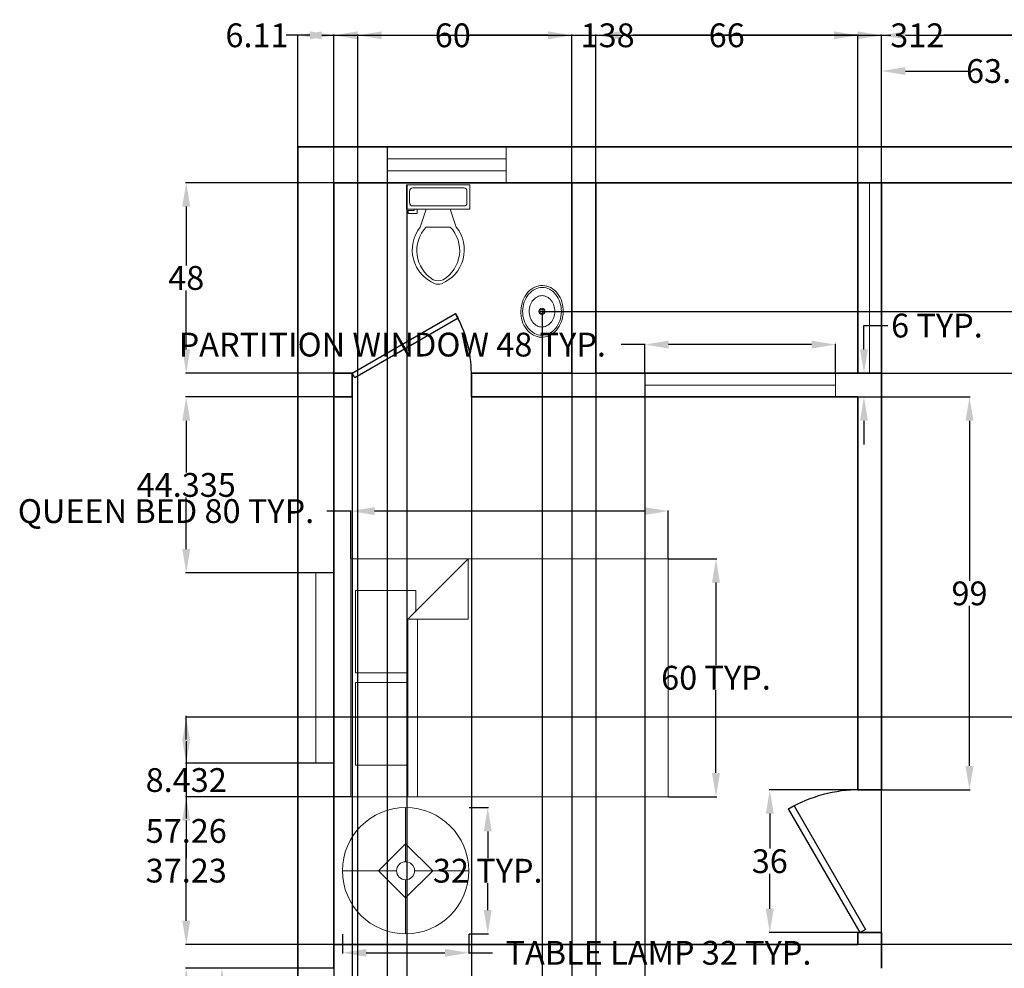
# Model space of a CAD drawing. Units: inches. Extents: x 351 to 774, y 111 to 703.
# Tile 5 of 6: x 351 to 599, y 464 to 703. Entities that reach past the tile are written whole.
import ezdxf

# ---------------------------------------------------------------- set-up
doc = ezdxf.new("R2010")
doc.units = ezdxf.units.IN
doc.header["$MEASUREMENT"] = 0
for name, color, linetype, lineweight in [('A-ANNO-DIMS', 2, 'Continuous', 18), ('A-DOOR', 3, 'Continuous', 25), ('A-FLOR-FIXT', 9, 'Continuous', 18), ('A-FURN', 8, 'Continuous', 18), ('A-GLAZ', 4, 'Continuous', 18), ('A-WALL', 7, 'Continuous', 35)]:
    doc.layers.add(name, color=color, linetype=linetype, lineweight=lineweight)
doc.styles.get("Standard").update_dxf_attribs({"font": 'arial.ttf'})
doc.dimstyles.get("Standard").update_dxf_attribs({"dimtxt": 6, "dimasz": 6, "dimexe": 0.18, "dimexo": 0.0625, "dimgap": 0.09, "dimtad": 0, "dimtih": 1, "dimtoh": 1, "dimdec": 0, "dimzin": 0, "dimdsep": 46, "dimlunit": 3, "dimtxsty": 'Standard', "dimcen": 0.09, "dimadec": 0, "dimazin": 0, "dimtfac": 1, "dimtdec": 0, "dimtofl": 0, "dimtmove": 0, "dimatfit": 3, "dimfxl": 1, "dimtolj": 1, "dimtzin": 0, "dimarcsym": 0})

# ---------------------------------------------------------------- blocks, each defined once
blk = doc.blocks.new('*U3')
for p, q in [((0, 0), (0, -6)), ((40, 0), (40, -6))]:
    blk.add_line(p, q)
blk.add_lwpolyline([(0, 0), (34.64, 20), (35.52, 18.48), (0.88, -1.52)], close=True)
blk.add_arc((0, 0), 40, 0, 30)
blk = doc.blocks.new('*U4')
for p, q in [((-40, 0), (-40, 6)), ((0, 0), (0, 6))]:
    blk.add_line(p, q)
blk.add_lwpolyline([(0, 0), (-34.64, -20), (-35.52, -18.48), (-0.88, 1.52)], close=True)
blk.add_arc((0, 0), 40, 180, 210)
blk = doc.blocks.new('Bed - Queen')
for p, q in [((0, -80.00003), (0, 0)), ((0, 0), (59.99999, 0)), ((59.99999, 0), (59.99999, -80.00003)), ((7.99999, -1.2), (28.79998, -1.2)), ((7.99999, -14.4), (7.99999, -1.2)), ((28.79998, -1.2), (28.79998, -14.4)), ((31.19999, -1.2), (51.99999, -1.2)), ((31.19999, -14.4), (31.19999, -1.2)), ((51.99999, -1.2), (51.99999, -16.4)), ((0, -14.4), (44.8, -14.4)), ((59.99999, -29.6), (44.8, -14.4)), ((44.8, -14.4), (44.8, -29.6)), ((44.8, -16.8), (0, -16.8)), ((51.99999, -16.4), (46.79936, -16.4)), ((44.8, -29.6), (59.99999, -29.6)), ((59.99999, -80.00003), (0, -80.00003))]:
    blk.add_line(p, q)
blk = doc.blocks.new('Lamp - Table')
for p, q in [((0, 7), (0, 1)), ((0, 3), (-3, 0)), ((3, 0), (0, 3)), ((-1, 0), (-7, 0)), ((-3, 0), (0, -3)), ((0, -3), (3, 0)), ((1, 0), (7, 0)), ((0, -1), (0, -7))]:
    blk.add_line(p, q)
for radius in [7, 1]:
    blk.add_circle((0, 0), radius)
blk = doc.blocks.new('Toilet - top')
for p, q in [((9.5, -6), (9.5, -2)), ((-10, -8.5), (-8, -8.5)), ((-10, -9.5), (-10, -8.5)), ((-7, -9.5), (-10, -9.5)), ((-8, -8.5), (-8, -8)), ((-7, -8), (-7, -9.5)), ((-4, -8), (-6, -14)), ((4, -8), (6, -14)), ((4, -14), (-4, -14))]:
    blk.add_line(p, q)
blk.add_lwpolyline([(10.5, -8), (10.5, 0), (-10.5, 0), (-10.5, -8)], close=True)
for points in [[(-9.5, -2), (-9.5, -6)], [(8.5, -1), (-8.5, -1)], [(-8.5, -7), (8.5, -7)]]:
    blk.add_lwpolyline(points)
for centre, radius, start, end in [((-8.62, -1.88), 0.884, 81.8699, 188.1301), ((8.62, -1.88), 0.884, 351.8699, 98.1301), ((-8.62, -6.12), 0.884, 171.8699, 278.1301), ((8.62, -6.12), 0.884, 261.8699, 8.1301), ((3.52, -21.58), 12.17, 141.4691, 247.9714), ((4.2, -21.82), 11.33, 136.3677, 238.9468), ((-3.52, -21.58), 12.17, 292.0284, 38.5307), ((-4.2, -21.82), 11.33, 301.053, 43.6321), ((0, -27.88), 4, 245.7318, 294.2682), ((0, -29), 4, 254.8605, 285.1395)]:
    blk.add_arc(centre, radius, start, end)
blk = doc.blocks.new('Sink - Oval top')
for p, q in [((-1, 0), (1, 0)), ((0, 1), (0, -1))]:
    blk.add_line(p, q)
for points in [[(-12.23, 0.39, 0.117634), (-11.46, -3.36, 0.104469), (-8.88, -6.8, 0.090016), (-5.08, -9.07, 0.08192), (-0.32, -10.02, 0.08192), (4.49, -9.38, 0.090016), (8.42, -7.36, 0.104469), (11.22, -4.09, 0.117634), (12.23, -0.39, 0.117634), (11.46, 3.36, 0.104469), (8.88, 6.8, 0.090016), (5.08, 9.07, 0.08192), (0.32, 10.02, 0.08192), (-4.49, 9.38, 0.090016), (-8.42, 7.36, 0.104469), (-11.22, 4.09, 0.117634)], [(-11.29, 0.16, 0.118622), (-10.52, -3.25, 0.104678), (-8.07, -6.36, 0.089562), (-4.54, -8.37, 0.081185), (-0.13, -9.15, 0.081185), (4.3, -8.49, 0.089562), (7.89, -6.58, 0.104678), (10.42, -3.55, 0.118622), (11.29, -0.16, 0.118622), (10.52, 3.25, 0.104678), (8.07, 6.36, 0.089562), (4.54, 8.37, 0.081185), (0.13, 9.15, 0.081185), (-4.3, 8.49, 0.089562), (-7.89, 6.58, 0.104678), (-10.42, 3.55, 0.118622)], [(-7.42, 0.08, 0.118283), (-6.91, -2.17, 0.104607), (-5.29, -4.21, 0.089718), (-2.97, -5.53, 0.081436), (-0.07, -6.04, 0.081436), (2.84, -5.59, 0.089718), (5.2, -4.33, 0.104607), (6.86, -2.32, 0.118283), (7.42, -0.08, 0.118283), (6.91, 2.17, 0.104607), (5.29, 4.21, 0.089718), (2.97, 5.53, 0.081436), (0.07, 6.04, 0.081436), (-2.84, 5.59, 0.089718), (-5.2, 4.33, 0.104607), (-6.86, 2.32, 0.118283)]]:
    blk.add_lwpolyline(points, format="xyb", close=True)
for radius in [1.5, 1]:
    blk.add_circle((0, 0), radius)
blk = doc.blocks.new('WIN-48IN-6IN-WALL')
blk.add_line((3, 48), (3, 0))
blk.add_lwpolyline([(0, 48), (6, 48), (6, 0), (0, 0)], close=True)
blk = doc.blocks.new('WIN-48IN-9IN-WALL')
blk.add_line((4.5, 48), (4.5, 0))
blk.add_lwpolyline([(0, 0), (9, 0), (9, 48), (0, 48)], close=True)
blk = doc.blocks.new('WIN-BATH-30IN-9IN-WALL')
for p, q in [((0, 0), (0, 9)), ((0, 9), (30, 9)), ((30, 9), (30, 0)), ((0, 6), (30, 6)), ((30, 3), (0, 3)), ((30, 0), (0, 0))]:
    blk.add_line(p, q)
blk = doc.blocks.new('*D22')
at = {"layer": 'A-ANNO-DIMS', "color": 0, "lineweight": -2, "transparency": 16777216}
for p, q in [((508.41, 621.44), (502.41, 621.44)), ((508.41, 614.3), (508.41, 621.62)), ((550.41, 621.44), (514.41, 621.44)), ((556.41, 614.3), (556.41, 621.62))]:
    blk.add_line(p, q, dxfattribs=at)
at = {"layer": 'A-ANNO-DIMS', "color": 0, "transparency": 16777216}
for points in [[(514.41, 622.44), (514.41, 620.44), (508.41, 621.44)], [(550.41, 622.44), (550.41, 620.44), (556.41, 621.44)]]:
    blk.add_solid(points, dxfattribs=at)
at = {"layer": 'Defpoints', "color": 0, "transparency": 16777216}
for p in [(508.41, 621.44), (508.41, 614.24), (556.41, 614.24)]:
    blk.add_point(p, dxfattribs=at)
at = {"layer": 'A-ANNO-DIMS', "color": 0, "transparency": 16777216, "insert": (444.8, 621.44), "char_height": 6, "attachment_point": 5}
blk.add_mtext('\\A1;PARTITION WINDOW 48 TYP.', dxfattribs=at)
blk = doc.blocks.new('*D23')
at = {"layer": 'A-ANNO-DIMS', "color": 0, "lineweight": -2, "transparency": 16777216}
for p, q in [((563.61, 620.24), (563.61, 626.24)), ((563.61, 626.24), (569.61, 626.24)), ((556.48, 614.24), (563.79, 614.24)), ((556.48, 608.24), (563.79, 608.24)), ((563.61, 602.24), (563.61, 596.24))]:
    blk.add_line(p, q, dxfattribs=at)
at = {"layer": 'A-ANNO-DIMS', "color": 0, "transparency": 16777216}
for points in [[(562.61, 620.24), (564.61, 620.24), (563.61, 614.24)], [(562.61, 602.24), (564.61, 602.24), (563.61, 608.24)]]:
    blk.add_solid(points, dxfattribs=at)
at = {"layer": 'Defpoints', "color": 0, "transparency": 16777216}
for p in [(556.41, 614.24), (563.61, 614.24), (556.41, 608.24)]:
    blk.add_point(p, dxfattribs=at)
at = {"layer": 'A-ANNO-DIMS', "color": 0, "transparency": 16777216, "insert": (581.99, 626.24), "char_height": 6, "attachment_point": 5}
blk.add_mtext('\\A1;6 TYP.', dxfattribs=at)
blk = doc.blocks.new('*D28')
at = {"layer": 'A-ANNO-DIMS', "color": 0, "lineweight": -2, "transparency": 16777216}
for p, q in [((432.23, 472.86), (432.23, 467.97)), ((464.06, 472.86), (464.06, 467.97)), ((438.23, 468.15), (458.06, 468.15)), ((464.06, 468.15), (470.06, 468.15))]:
    blk.add_line(p, q, dxfattribs=at)
at = {"layer": 'A-ANNO-DIMS', "color": 0, "transparency": 16777216}
for points in [[(438.23, 469.15), (438.23, 467.15), (432.23, 468.15)], [(458.06, 469.15), (458.06, 467.15), (464.06, 468.15)]]:
    blk.add_solid(points, dxfattribs=at)
at = {"layer": 'Defpoints', "color": 0, "transparency": 16777216}
for p in [(432.23, 472.92), (464.06, 472.92), (464.06, 468.15)]:
    blk.add_point(p, dxfattribs=at)
at = {"layer": 'A-ANNO-DIMS', "color": 0, "transparency": 16777216, "insert": (511.85, 468.15), "char_height": 6, "attachment_point": 5}
blk.add_mtext('\\A1;TABLE LAMP 32 TYP.', dxfattribs=at)
blk = doc.blocks.new('*D29')
at = {"layer": 'A-ANNO-DIMS', "color": 0, "lineweight": -2, "transparency": 16777216}
for p, q in [((464.12, 504.75), (469.02, 504.75)), ((468.84, 498.75), (468.84, 491.99)), ((468.84, 478.92), (468.84, 485.68)), ((464.12, 472.92), (469.02, 472.92))]:
    blk.add_line(p, q, dxfattribs=at)
at = {"layer": 'A-ANNO-DIMS', "color": 0, "transparency": 16777216}
for points in [[(467.84, 498.75), (469.84, 498.75), (468.84, 504.75)], [(467.84, 478.92), (469.84, 478.92), (468.84, 472.92)]]:
    blk.add_solid(points, dxfattribs=at)
at = {"layer": 'Defpoints', "color": 0, "transparency": 16777216}
for p in [(464.06, 504.75), (468.84, 504.75), (464.06, 472.92)]:
    blk.add_point(p, dxfattribs=at)
at = {"layer": 'A-ANNO-DIMS', "color": 0, "transparency": 16777216, "insert": (468.84, 488.84), "char_height": 6, "attachment_point": 5}
blk.add_mtext('\\A1;32 TYP.', dxfattribs=at)
blk = doc.blocks.new('*D34')
at = {"layer": 'A-ANNO-DIMS', "color": 0, "lineweight": -2, "transparency": 16777216}
for p, q in [((434.33, 579.48), (428.33, 579.48)), ((434.33, 567.54), (434.33, 579.66)), ((508.33, 579.48), (440.33, 579.48)), ((514.33, 567.54), (514.33, 579.66))]:
    blk.add_line(p, q, dxfattribs=at)
at = {"layer": 'A-ANNO-DIMS', "color": 0, "transparency": 16777216}
for points in [[(440.33, 580.48), (440.33, 578.48), (434.33, 579.48)], [(508.33, 580.48), (508.33, 578.48), (514.33, 579.48)]]:
    blk.add_solid(points, dxfattribs=at)
at = {"layer": 'Defpoints', "color": 0, "transparency": 16777216}
for p in [(434.33, 579.48), (434.33, 567.48), (514.33, 567.48)]:
    blk.add_point(p, dxfattribs=at)
at = {"layer": 'A-ANNO-DIMS', "color": 0, "transparency": 16777216, "insert": (387.79, 579.48), "char_height": 6, "attachment_point": 5}
blk.add_mtext('\\A1;QUEEN BED 80 TYP.', dxfattribs=at)
blk = doc.blocks.new('*D35')
at = {"layer": 'A-ANNO-DIMS', "color": 0, "lineweight": -2, "transparency": 16777216}
for p, q in [((514.39, 567.48), (526.51, 567.48)), ((526.33, 561.48), (526.33, 540.63)), ((526.33, 513.48), (526.33, 534.32)), ((514.39, 507.48), (526.51, 507.48))]:
    blk.add_line(p, q, dxfattribs=at)
at = {"layer": 'A-ANNO-DIMS', "color": 0, "transparency": 16777216}
for points in [[(525.33, 561.48), (527.33, 561.48), (526.33, 567.48)], [(525.33, 513.48), (527.33, 513.48), (526.33, 507.48)]]:
    blk.add_solid(points, dxfattribs=at)
at = {"layer": 'Defpoints', "color": 0, "transparency": 16777216}
for p in [(514.33, 567.48), (526.33, 567.48), (514.33, 507.48)]:
    blk.add_point(p, dxfattribs=at)
at = {"layer": 'A-ANNO-DIMS', "color": 0, "transparency": 16777216, "insert": (526.33, 537.48), "char_height": 6, "attachment_point": 5}
blk.add_mtext('\\A1;60 TYP.', dxfattribs=at)
blk = doc.blocks.new('*D46')
at = {"layer": 'A-ANNO-DIMS', "color": 0, "lineweight": -2, "transparency": 16777216}
for p, q in [((421.04, 671.3), (421.04, 699.57)), ((733.04, 671.3), (733.04, 699.57)), ((427.04, 699.39), (570.36, 699.39)), ((727.04, 699.39), (583.73, 699.39))]:
    blk.add_line(p, q, dxfattribs=at)
at = {"layer": 'A-ANNO-DIMS', "color": 0, "transparency": 16777216}
for points in [[(427.04, 700.39), (427.04, 698.39), (421.04, 699.39)], [(727.04, 700.39), (727.04, 698.39), (733.04, 699.39)]]:
    blk.add_solid(points, dxfattribs=at)
at = {"layer": 'Defpoints', "color": 0, "transparency": 16777216}
for p in [(733.04, 699.39), (421.04, 671.24), (733.04, 671.24)]:
    blk.add_point(p, dxfattribs=at)
at = {"layer": 'A-ANNO-DIMS', "color": 0, "transparency": 16777216, "insert": (577.04, 699.39), "char_height": 6, "attachment_point": 5}
blk.add_mtext('\\A1;312', dxfattribs=at)
blk = doc.blocks.new('*D48')
at = {"layer": 'A-ANNO-DIMS', "color": 0, "lineweight": -2, "transparency": 16777216}
for p, q in [((430.04, 662.3), (430.04, 699.57)), ((490.04, 662.3), (490.04, 699.57)), ((436.04, 699.39), (455.65, 699.39)), ((484.04, 699.39), (464.44, 699.39))]:
    blk.add_line(p, q, dxfattribs=at)
at = {"layer": 'A-ANNO-DIMS', "color": 0, "transparency": 16777216}
for points in [[(436.04, 700.39), (436.04, 698.39), (430.04, 699.39)], [(484.04, 700.39), (484.04, 698.39), (490.04, 699.39)]]:
    blk.add_solid(points, dxfattribs=at)
at = {"layer": 'Defpoints', "color": 0, "transparency": 16777216}
for p in [(490.04, 699.39), (430.04, 662.24), (490.04, 662.24)]:
    blk.add_point(p, dxfattribs=at)
at = {"layer": 'A-ANNO-DIMS', "color": 0, "transparency": 16777216, "insert": (460.04, 699.39), "char_height": 6, "attachment_point": 5}
blk.add_mtext('\\A1;60', dxfattribs=at)
blk = doc.blocks.new('*D49')
at = {"layer": 'A-ANNO-DIMS', "color": 0, "lineweight": -2, "transparency": 16777216}
for p, q in [((496.04, 662.3), (496.04, 699.57)), ((562.04, 662.3), (562.04, 699.57)), ((502.04, 699.39), (524.64, 699.39)), ((556.04, 699.39), (533.44, 699.39))]:
    blk.add_line(p, q, dxfattribs=at)
at = {"layer": 'A-ANNO-DIMS', "color": 0, "transparency": 16777216}
for points in [[(502.04, 700.39), (502.04, 698.39), (496.04, 699.39)], [(556.04, 700.39), (556.04, 698.39), (562.04, 699.39)]]:
    blk.add_solid(points, dxfattribs=at)
at = {"layer": 'Defpoints', "color": 0, "transparency": 16777216}
for p in [(562.04, 699.39), (496.04, 662.24), (562.04, 662.24)]:
    blk.add_point(p, dxfattribs=at)
at = {"layer": 'A-ANNO-DIMS', "color": 0, "transparency": 16777216, "insert": (529.04, 699.39), "char_height": 6, "attachment_point": 5}
blk.add_mtext('\\A1;66', dxfattribs=at)
blk = doc.blocks.new('*D50')
at = {"layer": 'A-ANNO-DIMS', "color": 0, "lineweight": -2, "transparency": 16777216}
for p, q in [((421.04, 671.18), (421.04, 114.91)), ((443.48, 671.18), (443.48, 114.91)), ((427.04, 115.09), (437.48, 115.09)), ((443.48, 115.09), (449.48, 115.09))]:
    blk.add_line(p, q, dxfattribs=at)
at = {"layer": 'A-ANNO-DIMS', "color": 0, "transparency": 16777216}
for points in [[(427.04, 116.09), (427.04, 114.09), (421.04, 115.09)], [(437.48, 116.09), (437.48, 114.09), (443.48, 115.09)]]:
    blk.add_solid(points, dxfattribs=at)
at = {"layer": 'Defpoints', "color": 0, "transparency": 16777216}
for p in [(421.04, 671.24), (443.48, 671.24), (443.48, 115.09)]:
    blk.add_point(p, dxfattribs=at)
at = {"layer": 'A-ANNO-DIMS', "color": 0, "transparency": 16777216, "insert": (462.06, 115.09), "char_height": 6, "attachment_point": 5}
blk.add_mtext('\\A1;22.434', dxfattribs=at)
blk = doc.blocks.new('*D51')
at = {"layer": 'A-ANNO-DIMS', "color": 0, "lineweight": -2, "transparency": 16777216}
for p, q in [((568.04, 662.3), (568.04, 690.57)), ((574.04, 690.39), (589.9, 690.39)), ((625.05, 690.39), (609.2, 690.39)), ((631.05, 662.3), (631.05, 690.57))]:
    blk.add_line(p, q, dxfattribs=at)
at = {"layer": 'A-ANNO-DIMS', "color": 0, "transparency": 16777216}
for points in [[(574.04, 691.39), (574.04, 689.39), (568.04, 690.39)], [(625.05, 691.39), (625.05, 689.39), (631.05, 690.39)]]:
    blk.add_solid(points, dxfattribs=at)
at = {"layer": 'Defpoints', "color": 0, "transparency": 16777216}
for p in [(631.05, 690.39), (568.04, 662.24), (631.05, 662.24)]:
    blk.add_point(p, dxfattribs=at)
at = {"layer": 'A-ANNO-DIMS', "color": 0, "transparency": 16777216, "insert": (599.55, 690.39), "char_height": 6, "attachment_point": 5}
blk.add_mtext('\\A1;63.01', dxfattribs=at)
blk = doc.blocks.new('*D52')
at = {"layer": 'A-ANNO-DIMS', "color": 0, "lineweight": -2, "transparency": 16777216}
for p, q in [((429.98, 662.24), (392.71, 662.24)), ((392.89, 656.24), (392.89, 641.4)), ((392.89, 620.24), (392.89, 635.09)), ((429.98, 614.24), (392.71, 614.24))]:
    blk.add_line(p, q, dxfattribs=at)
at = {"layer": 'A-ANNO-DIMS', "color": 0, "transparency": 16777216}
for points in [[(391.89, 656.24), (393.89, 656.24), (392.89, 662.24)], [(391.89, 620.24), (393.89, 620.24), (392.89, 614.24)]]:
    blk.add_solid(points, dxfattribs=at)
at = {"layer": 'Defpoints', "color": 0, "transparency": 16777216}
for p in [(392.89, 662.24), (430.04, 662.24), (430.04, 614.24)]:
    blk.add_point(p, dxfattribs=at)
at = {"layer": 'A-ANNO-DIMS', "color": 0, "transparency": 16777216, "insert": (392.89, 638.24), "char_height": 6, "attachment_point": 5}
blk.add_mtext('\\A1;48', dxfattribs=at)
blk = doc.blocks.new('*D53')
at = {"layer": 'A-ANNO-DIMS', "color": 0, "lineweight": -2, "transparency": 16777216}
for p, q in [((434.27, 507.48), (392.71, 507.48)), ((392.89, 501.48), (392.89, 492.01)), ((392.89, 476.24), (392.89, 485.7)), ((429.98, 470.24), (392.71, 470.24))]:
    blk.add_line(p, q, dxfattribs=at)
at = {"layer": 'A-ANNO-DIMS', "color": 0, "transparency": 16777216}
for points in [[(391.89, 501.48), (393.89, 501.48), (392.89, 507.48)], [(391.89, 476.24), (393.89, 476.24), (392.89, 470.24)]]:
    blk.add_solid(points, dxfattribs=at)
at = {"layer": 'Defpoints', "color": 0, "transparency": 16777216}
for p in [(392.89, 507.48), (434.33, 507.48), (430.04, 470.24)]:
    blk.add_point(p, dxfattribs=at)
at = {"layer": 'A-ANNO-DIMS', "color": 0, "transparency": 16777216, "insert": (392.89, 488.86), "char_height": 6, "attachment_point": 5}
blk.add_mtext('\\A1;37.23', dxfattribs=at)
blk = doc.blocks.new('*D54')
at = {"layer": 'A-ANNO-DIMS', "color": 0, "lineweight": -2, "transparency": 16777216}
for p, q in [((429.98, 608.24), (392.71, 608.24)), ((392.89, 602.24), (392.89, 589.23)), ((392.89, 569.91), (392.89, 582.92)), ((429.98, 563.91), (392.71, 563.91))]:
    blk.add_line(p, q, dxfattribs=at)
at = {"layer": 'A-ANNO-DIMS', "color": 0, "transparency": 16777216}
for points in [[(391.89, 602.24), (393.89, 602.24), (392.89, 608.24)], [(391.89, 569.91), (393.89, 569.91), (392.89, 563.91)]]:
    blk.add_solid(points, dxfattribs=at)
at = {"layer": 'Defpoints', "color": 0, "transparency": 16777216}
for p in [(392.89, 608.24), (430.04, 608.24), (430.04, 563.91)]:
    blk.add_point(p, dxfattribs=at)
at = {"layer": 'A-ANNO-DIMS', "color": 0, "transparency": 16777216, "insert": (392.89, 586.07), "char_height": 6, "attachment_point": 5}
blk.add_mtext('\\A1;44.335', dxfattribs=at)
blk = doc.blocks.new('*D56')
at = {"layer": 'A-ANNO-DIMS', "color": 0, "lineweight": -2, "transparency": 16777216}
for p, q in [((429.98, 464.24), (401.71, 464.24)), ((401.89, 458.24), (401.89, 404.4)), ((401.89, 344.24), (401.89, 398.09)), ((429.98, 338.24), (401.71, 338.24))]:
    blk.add_line(p, q, dxfattribs=at)
at = {"layer": 'A-ANNO-DIMS', "color": 0, "transparency": 16777216}
for points in [[(400.89, 458.24), (402.89, 458.24), (401.89, 464.24)], [(400.89, 344.24), (402.89, 344.24), (401.89, 338.24)]]:
    blk.add_solid(points, dxfattribs=at)
at = {"layer": 'Defpoints', "color": 0, "transparency": 16777216}
for p in [(401.89, 464.24), (430.04, 464.24), (430.04, 338.24)]:
    blk.add_point(p, dxfattribs=at)
at = {"layer": 'A-ANNO-DIMS', "color": 0, "transparency": 16777216, "insert": (401.89, 401.24), "char_height": 6, "attachment_point": 5}
blk.add_mtext('\\A1;126', dxfattribs=at)
blk = doc.blocks.new('*D64')
at = {"layer": 'A-ANNO-DIMS', "color": 0, "lineweight": -2, "transparency": 16777216}
for p, q in [((663.98, 527.5), (392.71, 527.5)), ((392.89, 521.5), (392.89, 502.02)), ((392.89, 476.24), (392.89, 495.72)), ((663.98, 470.24), (392.71, 470.24))]:
    blk.add_line(p, q, dxfattribs=at)
at = {"layer": 'A-ANNO-DIMS', "color": 0, "transparency": 16777216}
for points in [[(391.89, 521.5), (393.89, 521.5), (392.89, 527.5)], [(391.89, 476.24), (393.89, 476.24), (392.89, 470.24)]]:
    blk.add_solid(points, dxfattribs=at)
at = {"layer": 'Defpoints', "color": 0, "transparency": 16777216}
for p in [(392.89, 527.5), (664.04, 527.5), (664.04, 470.24)]:
    blk.add_point(p, dxfattribs=at)
at = {"layer": 'A-ANNO-DIMS', "color": 0, "transparency": 16777216, "insert": (392.89, 498.87), "char_height": 6, "attachment_point": 5}
blk.add_mtext('\\A1;57.26', dxfattribs=at)
blk = doc.blocks.new('*D70')
at = {"layer": 'A-ANNO-DIMS', "color": 0, "lineweight": -2, "transparency": 16777216}
for p, q in [((430.04, 614.18), (430.04, 114.91)), ((434.71, 614.18), (434.71, 114.91)), ((424.04, 115.09), (418.04, 115.09)), ((440.71, 115.09), (446.71, 115.09))]:
    blk.add_line(p, q, dxfattribs=at)
at = {"layer": 'A-ANNO-DIMS', "color": 0, "transparency": 16777216}
for points in [[(424.04, 116.09), (424.04, 114.09), (430.04, 115.09)], [(440.71, 116.09), (440.71, 114.09), (434.71, 115.09)]]:
    blk.add_solid(points, dxfattribs=at)
at = {"layer": 'Defpoints', "color": 0, "transparency": 16777216}
for p in [(430.04, 614.24), (434.71, 614.24), (434.71, 115.09)]:
    blk.add_point(p, dxfattribs=at)
at = {"layer": 'A-ANNO-DIMS', "color": 0, "transparency": 16777216, "insert": (457.05, 115.09), "char_height": 6, "attachment_point": 5}
blk.add_mtext('\\A1;4.669', dxfattribs=at)
blk = doc.blocks.new('*D71')
at = {"layer": 'A-ANNO-DIMS', "color": 0, "lineweight": -2, "transparency": 16777216}
for p, q in [((434.71, 614.18), (434.71, 114.91)), ((464.71, 614.18), (464.71, 114.91)), ((440.71, 115.09), (445.34, 115.09)), ((458.71, 115.09), (454.09, 115.09))]:
    blk.add_line(p, q, dxfattribs=at)
at = {"layer": 'A-ANNO-DIMS', "color": 0, "transparency": 16777216}
for points in [[(440.71, 116.09), (440.71, 114.09), (434.71, 115.09)], [(458.71, 116.09), (458.71, 114.09), (464.71, 115.09)]]:
    blk.add_solid(points, dxfattribs=at)
at = {"layer": 'Defpoints', "color": 0, "transparency": 16777216}
for p in [(434.71, 614.24), (464.71, 614.24), (464.71, 115.09)]:
    blk.add_point(p, dxfattribs=at)
at = {"layer": 'A-ANNO-DIMS', "color": 0, "transparency": 16777216, "insert": (449.71, 115.09), "char_height": 6, "attachment_point": 5}
blk.add_mtext('\\A1;30', dxfattribs=at)
blk = doc.blocks.new('*D72')
at = {"layer": 'A-ANNO-DIMS', "color": 0, "lineweight": -2, "transparency": 16777216}
for p, q in [((567.98, 509.24), (539.71, 509.24)), ((539.89, 503.24), (539.89, 494.4)), ((539.89, 479.24), (539.89, 488.09)), ((567.98, 473.24), (539.71, 473.24))]:
    blk.add_line(p, q, dxfattribs=at)
at = {"layer": 'A-ANNO-DIMS', "color": 0, "transparency": 16777216}
for points in [[(538.89, 503.24), (540.89, 503.24), (539.89, 509.24)], [(538.89, 479.24), (540.89, 479.24), (539.89, 473.24)]]:
    blk.add_solid(points, dxfattribs=at)
at = {"layer": 'Defpoints', "color": 0, "transparency": 16777216}
for p in [(539.89, 509.24), (568.04, 509.24), (568.04, 473.24)]:
    blk.add_point(p, dxfattribs=at)
at = {"layer": 'A-ANNO-DIMS', "color": 0, "transparency": 16777216, "insert": (539.89, 491.24), "char_height": 6, "attachment_point": 5}
blk.add_mtext('\\A1;36', dxfattribs=at)
blk = doc.blocks.new('*D73')
at = {"layer": 'A-ANNO-DIMS', "color": 0, "lineweight": -2, "transparency": 16777216}
for p, q in [((562.11, 608.24), (590.37, 608.24)), ((590.19, 602.24), (590.19, 561.9)), ((590.19, 515.24), (590.19, 555.59)), ((562.11, 509.24), (590.37, 509.24))]:
    blk.add_line(p, q, dxfattribs=at)
at = {"layer": 'A-ANNO-DIMS', "color": 0, "transparency": 16777216}
for points in [[(589.19, 602.24), (591.19, 602.24), (590.19, 608.24)], [(589.19, 515.24), (591.19, 515.24), (590.19, 509.24)]]:
    blk.add_solid(points, dxfattribs=at)
at = {"layer": 'Defpoints', "color": 0, "transparency": 16777216}
for p in [(562.04, 608.24), (562.04, 509.24), (590.19, 509.24)]:
    blk.add_point(p, dxfattribs=at)
at = {"layer": 'A-ANNO-DIMS', "color": 0, "transparency": 16777216, "insert": (590.19, 558.74), "char_height": 6, "attachment_point": 5}
blk.add_mtext('\\A1;99', dxfattribs=at)
blk = doc.blocks.new('*D79')
at = {"layer": 'A-ANNO-DIMS', "color": 0, "lineweight": -2, "transparency": 16777216}
for p, q in [((430.04, 464.3), (430.04, 699.57)), ((568.04, 464.3), (568.04, 699.57)), ((436.04, 699.39), (492.6, 699.39)), ((562.04, 699.39), (505.49, 699.39))]:
    blk.add_line(p, q, dxfattribs=at)
at = {"layer": 'A-ANNO-DIMS', "color": 0, "transparency": 16777216}
for points in [[(436.04, 700.39), (436.04, 698.39), (430.04, 699.39)], [(562.04, 700.39), (562.04, 698.39), (568.04, 699.39)]]:
    blk.add_solid(points, dxfattribs=at)
at = {"layer": 'Defpoints', "color": 0, "transparency": 16777216}
for p in [(568.04, 699.39), (430.04, 464.24), (568.04, 464.24)]:
    blk.add_point(p, dxfattribs=at)
at = {"layer": 'A-ANNO-DIMS', "color": 0, "transparency": 16777216, "insert": (499.04, 699.39), "char_height": 6, "attachment_point": 5}
blk.add_mtext('\\A1;138', dxfattribs=at)
blk = doc.blocks.new('*D80')
at = {"layer": 'A-ANNO-DIMS', "color": 0, "lineweight": -2, "transparency": 16777216}
for p, q in [((568.04, 464.3), (568.04, 699.57)), ((658.04, 464.3), (658.04, 699.57)), ((574.04, 699.39), (608.67, 699.39)), ((652.04, 699.39), (617.42, 699.39))]:
    blk.add_line(p, q, dxfattribs=at)
at = {"layer": 'A-ANNO-DIMS', "color": 0, "transparency": 16777216}
for points in [[(574.04, 700.39), (574.04, 698.39), (568.04, 699.39)], [(652.04, 700.39), (652.04, 698.39), (658.04, 699.39)]]:
    blk.add_solid(points, dxfattribs=at)
at = {"layer": 'Defpoints', "color": 0, "transparency": 16777216}
for p in [(658.04, 699.39), (568.04, 464.24), (658.04, 464.24)]:
    blk.add_point(p, dxfattribs=at)
at = {"layer": 'A-ANNO-DIMS', "color": 0, "transparency": 16777216, "insert": (613.04, 699.39), "char_height": 6, "attachment_point": 5}
blk.add_mtext('\\A1;90', dxfattribs=at)
blk = doc.blocks.new('*D91')
at = {"layer": 'A-ANNO-DIMS', "color": 0, "lineweight": -2, "transparency": 16777216}
for p, q in [((496.04, 614.18), (496.04, 114.91)), ((508.41, 614.18), (508.41, 114.91)), ((502.04, 115.09), (502.41, 115.09)), ((508.41, 115.09), (514.41, 115.09))]:
    blk.add_line(p, q, dxfattribs=at)
at = {"layer": 'A-ANNO-DIMS', "color": 0, "transparency": 16777216}
for points in [[(502.04, 116.09), (502.04, 114.09), (496.04, 115.09)], [(502.41, 116.09), (502.41, 114.09), (508.41, 115.09)]]:
    blk.add_solid(points, dxfattribs=at)
at = {"layer": 'Defpoints', "color": 0, "transparency": 16777216}
for p in [(496.04, 614.24), (508.41, 614.24), (508.41, 115.09)]:
    blk.add_point(p, dxfattribs=at)
at = {"layer": 'A-ANNO-DIMS', "color": 0, "transparency": 16777216, "insert": (526.65, 115.09), "char_height": 6, "attachment_point": 5}
blk.add_mtext('\\A1;12.372', dxfattribs=at)
blk = doc.blocks.new('*D94')
at = {"layer": 'A-ANNO-DIMS', "color": 0, "lineweight": -2, "transparency": 16777216}
for p, q in [((430.04, 464.3), (430.04, 699.57)), ((436.15, 432.88), (436.15, 699.57)), ((424.04, 699.39), (418.04, 699.39)), ((442.15, 699.39), (448.15, 699.39))]:
    blk.add_line(p, q, dxfattribs=at)
at = {"layer": 'A-ANNO-DIMS', "color": 0, "transparency": 16777216}
for points in [[(424.04, 700.39), (424.04, 698.39), (430.04, 699.39)], [(442.15, 700.39), (442.15, 698.39), (436.15, 699.39)]]:
    blk.add_solid(points, dxfattribs=at)
at = {"layer": 'Defpoints', "color": 0, "transparency": 16777216}
for p in [(430.04, 699.39), (430.04, 464.24), (436.15, 432.82)]:
    blk.add_point(p, dxfattribs=at)
at = {"layer": 'A-ANNO-DIMS', "color": 0, "transparency": 16777216, "insert": (410.72, 699.39), "char_height": 6, "attachment_point": 5}
blk.add_mtext('\\A1;6.11', dxfattribs=at)
blk = doc.blocks.new('*D95')
at = {"layer": 'A-ANNO-DIMS', "color": 0, "lineweight": -2, "transparency": 16777216}
for p, q in [((429.98, 464.24), (392.71, 464.24)), ((392.89, 458.24), (392.89, 451.69)), ((392.89, 438.82), (392.89, 445.38)), ((436.09, 432.82), (392.71, 432.82))]:
    blk.add_line(p, q, dxfattribs=at)
at = {"layer": 'A-ANNO-DIMS', "color": 0, "transparency": 16777216}
for points in [[(391.89, 458.24), (393.89, 458.24), (392.89, 464.24)], [(391.89, 438.82), (393.89, 438.82), (392.89, 432.82)]]:
    blk.add_solid(points, dxfattribs=at)
at = {"layer": 'Defpoints', "color": 0, "transparency": 16777216}
for p in [(430.04, 464.24), (392.89, 432.82), (436.15, 432.82)]:
    blk.add_point(p, dxfattribs=at)
at = {"layer": 'A-ANNO-DIMS', "color": 0, "transparency": 16777216, "insert": (392.89, 448.53), "char_height": 6, "attachment_point": 5}
blk.add_mtext('\\A1;31.42', dxfattribs=at)
blk = doc.blocks.new('*D98')
at = {"layer": 'A-ANNO-DIMS', "color": 0, "lineweight": -2, "transparency": 16777216}
for p, q in [((482.58, 629.82), (761.37, 629.82)), ((761.19, 623.82), (761.19, 620.24)), ((490.11, 614.24), (761.37, 614.24)), ((761.19, 614.24), (761.19, 608.24)), ((761.19, 608.24), (755.19, 608.24))]:
    blk.add_line(p, q, dxfattribs=at)
at = {"layer": 'A-ANNO-DIMS', "color": 0, "transparency": 16777216}
for points in [[(760.19, 623.82), (762.19, 623.82), (761.19, 629.82)], [(760.19, 620.24), (762.19, 620.24), (761.19, 614.24)]]:
    blk.add_solid(points, dxfattribs=at)
at = {"layer": 'Defpoints', "color": 0, "transparency": 16777216}
for p in [(482.51, 629.82), (490.04, 614.24), (761.19, 614.24)]:
    blk.add_point(p, dxfattribs=at)
at = {"layer": 'A-ANNO-DIMS', "color": 0, "transparency": 16777216, "insert": (742.93, 608.24), "char_height": 6, "attachment_point": 5}
blk.add_mtext('\\A1;15.576', dxfattribs=at)
blk = doc.blocks.new('*D99')
at = {"layer": 'A-ANNO-DIMS', "color": 0, "lineweight": -2, "transparency": 16777216}
for p, q in [((482.51, 629.76), (482.51, 114.91)), ((490.04, 614.18), (490.04, 114.91)), ((476.51, 115.09), (470.51, 115.09)), ((496.04, 115.09), (502.04, 115.09))]:
    blk.add_line(p, q, dxfattribs=at)
at = {"layer": 'A-ANNO-DIMS', "color": 0, "transparency": 16777216}
for points in [[(476.51, 116.09), (476.51, 114.09), (482.51, 115.09)], [(496.04, 116.09), (496.04, 114.09), (490.04, 115.09)]]:
    blk.add_solid(points, dxfattribs=at)
at = {"layer": 'Defpoints', "color": 0, "transparency": 16777216}
for p in [(482.51, 629.82), (490.04, 614.24), (490.04, 115.09)]:
    blk.add_point(p, dxfattribs=at)
at = {"layer": 'A-ANNO-DIMS', "color": 0, "transparency": 16777216, "insert": (512.24, 115.09), "char_height": 6, "attachment_point": 5}
blk.add_mtext('\\A1;7.528', dxfattribs=at)
blk = doc.blocks.new('*D100')
at = {"layer": 'A-ANNO-DIMS', "color": 0, "lineweight": -2, "transparency": 16777216}
for p, q in [((430.04, 662.18), (430.04, 114.91)), ((448.42, 661.61), (448.42, 114.91)), ((430.04, 115.09), (424.04, 115.09)), ((442.42, 115.09), (436.04, 115.09))]:
    blk.add_line(p, q, dxfattribs=at)
at = {"layer": 'A-ANNO-DIMS', "color": 0, "transparency": 16777216}
for points in [[(436.04, 116.09), (436.04, 114.09), (430.04, 115.09)], [(442.42, 116.09), (442.42, 114.09), (448.42, 115.09)]]:
    blk.add_solid(points, dxfattribs=at)
at = {"layer": 'Defpoints', "color": 0, "transparency": 16777216}
for p in [(430.04, 662.24), (448.42, 661.68), (430.04, 115.09)]:
    blk.add_point(p, dxfattribs=at)
at = {"layer": 'A-ANNO-DIMS', "color": 0, "transparency": 16777216, "insert": (411.78, 115.09), "char_height": 6, "attachment_point": 5}
blk.add_mtext('\\A1;18.373', dxfattribs=at)
blk = doc.blocks.new('*D105')
at = {"layer": 'A-ANNO-DIMS', "color": 0, "lineweight": -2, "transparency": 16777216}
for p, q in [((392.89, 521.91), (392.89, 527.91)), ((429.98, 515.91), (392.71, 515.91)), ((434.27, 507.48), (392.71, 507.48)), ((392.89, 501.48), (392.89, 495.48))]:
    blk.add_line(p, q, dxfattribs=at)
at = {"layer": 'A-ANNO-DIMS', "color": 0, "transparency": 16777216}
for points in [[(391.89, 521.91), (393.89, 521.91), (392.89, 515.91)], [(391.89, 501.48), (393.89, 501.48), (392.89, 507.48)]]:
    blk.add_solid(points, dxfattribs=at)
at = {"layer": 'Defpoints', "color": 0, "transparency": 16777216}
for p in [(392.89, 515.91), (430.04, 515.91), (434.33, 507.48)]:
    blk.add_point(p, dxfattribs=at)
at = {"layer": 'A-ANNO-DIMS', "color": 0, "transparency": 16777216, "insert": (392.89, 511.69), "char_height": 6, "attachment_point": 5}
blk.add_mtext('\\A1;8.432', dxfattribs=at)

msp = doc.modelspace()

# ---------------------------------------------------------------- linework, layer by layer
at = {"layer": 'A-WALL'}
for p, q in [((430.043, 662.2421), (724.043, 662.2421)), ((430.043, 470.2421), (430.043, 662.2421)), ((490.043, 614.2421), (490.043, 662.2421)), ((496.043, 614.2421), (496.043, 662.2421)), ((562.043, 614.2421), (562.043, 662.2421)), ((568.043, 509.2421), (568.043, 662.2421)), ((430.043, 614.2421), (434.7119, 614.2421)), ((464.7119, 614.2421), (490.043, 614.2421)), ((496.043, 614.2421), (568.043, 614.2421)), ((430.043, 608.2421), (434.7119, 608.2421)), ((464.7119, 608.2421), (562.043, 608.2421)), ((562.043, 509.2421), (562.043, 608.2421)), ((562.043, 509.2421), (568.043, 509.2421)), ((562.043, 473.2421), (568.043, 473.2421)), ((562.043, 470.2421), (562.043, 473.2421)), ((568.043, 470.2421), (568.043, 473.2421)), ((430.043, 470.2421), (562.043, 470.2421)), ((568.043, 470.2421), (568.043, 464.2421))]:
    msp.add_line(p, q, dxfattribs=at)
for points in [[(436.7781, 143.2421), (421.043, 143.2421), (421.043, 671.2421), (733.043, 671.2421), (733.043, 143.2421), (562.043, 143.2421)], [(434.7119, 614.2421), (434.7119, 608.2421)], [(464.7119, 608.2421), (464.7119, 614.2421)]]:
    msp.add_lwpolyline(points, dxfattribs=at)

# ---------------------------------------------------------------- block references
at = {"layer": 'A-DOOR', "xscale": 0.75, "yscale": 0.75, "zscale": 0.75}
msp.add_blockref('*U3', (434.7119, 614.2421), dxfattribs=at)
at = {"layer": 'A-DOOR', "xscale": 0.8999999999999985, "yscale": 0.8999999999999985, "zscale": 0.8999999999999985, "rotation": 270}
msp.add_blockref('*U4', (562.643, 473.2421), dxfattribs=at)
at = {"layer": 'A-FLOR-FIXT', "xscale": 0.7577391478424742, "yscale": 0.7577391478424742, "zscale": 0.7577391478424742}
msp.add_blockref('Toilet - top', (456.3722, 661.6763), dxfattribs=at)
at = {"layer": 'A-FLOR-FIXT', "xscale": 0.53295403104476, "yscale": 0.53295403104476, "zscale": 0.53295403104476, "rotation": 270}
msp.add_blockref('Sink - Oval top', (482.5147, 629.8184), dxfattribs=at)
at = {"layer": 'A-FURN', "rotation": 90}
msp.add_blockref('Bed - Queen', (434.3315, 507.4751), dxfattribs=at)
at = {"layer": 'A-FURN', "xscale": 2.273403864676251, "yscale": 2.273403864676251, "zscale": 2.273403864676251}
msp.add_blockref('Lamp - Table', (448.1476, 488.8373), dxfattribs=at)
at = {"layer": 'A-GLAZ'}
for name, p in [('WIN-BATH-30IN-9IN-WALL', (443.4772, 662.2421)), ('WIN-48IN-6IN-WALL', (562.043, 614.2421)), ('WIN-48IN-9IN-WALL', (421.043, 515.9073))]:
    msp.add_blockref(name, p, dxfattribs=at)
at = {"layer": 'A-GLAZ', "rotation": 90.00000000000003}
msp.add_blockref('WIN-48IN-6IN-WALL', (556.4146, 608.2421), dxfattribs=at)

# ---------------------------------------------------------------- dimensions: what is measured, and where the dimension line sits
at = {"layer": 'A-ANNO-DIMS'}
for base, p1, p2, override, picture, middle in [((430.043, 699.3921), (436.1529, 432.8215), (430.043, 464.2421), {"dimdec": 2, "dimlfac": 1, "dimrnd": 0, "dimzin": 0, "dimdsep": 46, "dimlunit": 2}, '*D94', (410.7231, 699.3921)), ((733.043, 699.3921), (421.043, 671.2421), (733.043, 671.2421), {"dimdec": 0, "dimlfac": 1, "dimrnd": 0, "dimzin": 0, "dimdsep": 46, "dimlunit": 2}, '*D46', (577.043, 699.3921)), ((490.043, 699.3921), (430.043, 662.2421), (490.043, 662.2421), {"dimdec": 0, "dimlfac": 1, "dimrnd": 0, "dimzin": 0, "dimdsep": 46, "dimlunit": 2}, '*D48', (460.043, 699.3921)), ((568.043, 699.3921), (430.043, 464.2421), (568.043, 464.2421), {"dimdec": 0, "dimlfac": 1, "dimrnd": 0, "dimzin": 0, "dimdsep": 46, "dimlunit": 2}, '*D79', (499.043, 699.3921)), ((562.043, 699.3921), (496.043, 662.2421), (562.043, 662.2421), {"dimdec": 0, "dimlfac": 1, "dimrnd": 0, "dimzin": 0, "dimdsep": 46, "dimlunit": 2}, '*D49', (529.043, 699.3921)), ((658.043, 699.3921), (568.043, 464.2421), (658.043, 464.2421), {"dimdec": 0, "dimlfac": 1, "dimrnd": 0, "dimzin": 0, "dimdsep": 46, "dimlunit": 2}, '*D80', (613.043, 699.3921)), ((631.0513, 690.3921), (568.043, 662.2421), (631.0513, 662.2421), {"dimdec": 2, "dimlfac": 1, "dimrnd": 0, "dimzin": 0, "dimdsep": 46, "dimlunit": 2}, '*D51', (599.5471, 690.3921)), ((443.4772, 115.0921), (421.043, 671.2421), (443.4772, 671.2421), {"dimdec": 3, "dimlfac": 1, "dimrnd": 0, "dimzin": 0, "dimdsep": 46, "dimlunit": 2}, '*D50', (462.0604, 115.0921)), ((430.043, 115.0921), (448.416, 661.6763), (430.043, 662.2421), {"dimdec": 3, "dimlfac": 1, "dimrnd": 0, "dimzin": 0, "dimdsep": 46, "dimlunit": 2}, '*D100', (411.7811, 115.0921)), ((490.043, 115.0921), (482.5147, 629.8184), (490.043, 614.2421), {"dimdec": 3, "dimlfac": 1, "dimrnd": 0, "dimzin": 0, "dimdsep": 46, "dimlunit": 2}, '*D99', (512.2381, 115.0921)), ((434.7119, 115.0921), (430.043, 614.2421), (434.7119, 614.2421), {"dimdec": 3, "dimlfac": 1, "dimrnd": 0, "dimzin": 0, "dimdsep": 46, "dimlunit": 2}, '*D70', (457.0522, 115.0921)), ((464.7119, 115.0921), (434.7119, 614.2421), (464.7119, 614.2421), {"dimdec": 0, "dimlfac": 1, "dimrnd": 0, "dimzin": 0, "dimdsep": 46, "dimlunit": 2}, '*D71', (449.7119, 115.0921)), ((508.4146, 115.0921), (496.043, 614.2421), (508.4146, 614.2421), {"dimdec": 3, "dimlfac": 1, "dimrnd": 0, "dimzin": 0, "dimdsep": 46, "dimlunit": 2}, '*D91', (526.6458, 115.0921))]:
    dim = msp.add_linear_dim(base=base, p1=p1, p2=p2, dimstyle='Standard', override=override, dxfattribs=at)
    dim.commit()
    dim.dimension.update_dxf_attribs({"geometry": picture, "text_midpoint": middle})
for base, p1, p2, angle, override, picture, middle in [((392.893, 662.2421), (430.043, 614.2421), (430.043, 662.2421), 90, {"dimdec": 0, "dimlfac": 1, "dimrnd": 0, "dimzin": 0, "dimdsep": 46, "dimlunit": 2}, '*D52', (392.893, 638.2421)), ((761.193, 614.2421), (482.5147, 629.8184), (490.043, 614.2421), 90, {"dimdec": 3, "dimlfac": 1, "dimrnd": 0, "dimzin": 0, "dimdsep": 46, "dimlunit": 2}, '*D98', (742.9332, 608.2421)), ((392.893, 608.2421), (430.043, 563.9073), (430.043, 608.2421), 90, {"dimdec": 3, "dimlfac": 1, "dimrnd": 0, "dimzin": 0, "dimdsep": 46, "dimlunit": 2}, '*D54', (392.893, 586.0747)), ((590.193, 509.2421), (562.043, 608.2421), (562.043, 509.2421), 270, {"dimdec": 0, "dimlfac": 1, "dimrnd": 0, "dimzin": 0, "dimdsep": 46, "dimlunit": 2}, '*D73', (590.193, 558.7421)), ((392.893, 515.9073), (434.3315, 507.4751), (430.043, 515.9073), 90, {"dimdec": 3, "dimlfac": 1, "dimrnd": 0, "dimzin": 0, "dimdsep": 46, "dimlunit": 2}, '*D105', (392.893, 511.6912)), ((392.893, 527.5), (664.043, 470.2421), (664.043, 527.5), 90, {"dimdec": 2, "dimlfac": 1, "dimrnd": 0, "dimzin": 0, "dimdsep": 46, "dimlunit": 2}, '*D64', (392.893, 498.871)), ((539.893, 509.2421), (568.043, 473.2421), (568.043, 509.2421), 90, {"dimdec": 0, "dimlfac": 1, "dimrnd": 0, "dimzin": 0, "dimdsep": 46, "dimlunit": 2}, '*D72', (539.893, 491.2421)), ((392.893, 507.4751), (430.043, 470.2421), (434.3315, 507.4751), 90, {"dimdec": 2, "dimlfac": 1, "dimrnd": 0, "dimzin": 0, "dimdsep": 46, "dimlunit": 2}, '*D53', (392.893, 488.8586)), ((392.893, 432.8215), (430.043, 464.2421), (436.1529, 432.8215), 90, {"dimdec": 2, "dimlfac": 1, "dimrnd": 0, "dimzin": 0, "dimdsep": 46, "dimlunit": 2}, '*D95', (392.893, 448.5318)), ((401.893, 464.2421), (430.043, 338.2421), (430.043, 464.2421), 90, {"dimdec": 0, "dimlfac": 1, "dimrnd": 0, "dimzin": 0, "dimdsep": 46, "dimlunit": 2}, '*D56', (401.893, 401.2421))]:
    dim = msp.add_linear_dim(base=base, p1=p1, p2=p2, angle=angle, dimstyle='Standard', override=override, dxfattribs=at)
    dim.commit()
    dim.dimension.update_dxf_attribs({"geometry": picture, "text_midpoint": middle})
for base, p1, p2, angle, text, picture, middle in [((508.4146, 621.4421), (556.4146, 614.2421), (508.4146, 614.2421), 180, 'PARTITION WINDOW <> TYP.', '*D22', (444.8008, 621.4421)), ((563.6146, 614.2421), (556.4146, 608.2421), (556.4146, 614.2421), 90, '<> TYP.', '*D23', (581.9932, 626.2421)), ((434.3315, 579.4751), (514.3315, 567.4751), (434.3315, 567.4751), 180, 'QUEEN BED <> TYP.', '*D34', (387.7947, 579.4751)), ((526.3315, 567.4751), (514.3315, 507.4751), (514.3315, 567.4751), 90, '<> TYP.', '*D35', (526.3315, 537.4751)), ((468.8356, 504.7511), (464.0615, 472.9235), (464.0615, 504.7511), 90, '<> TYP.', '*D29', (468.8356, 488.8373))]:
    dim = msp.add_linear_dim(base=base, p1=p1, p2=p2, angle=angle, text=text, dimstyle='Standard', override={"dimdec": 0, "dimlfac": 1, "dimrnd": 0, "dimzin": 0, "dimdsep": 46, "dimlunit": 2}, dxfattribs=at)
    dim.commit()
    dim.dimension.update_dxf_attribs({"geometry": picture, "text_midpoint": middle})
dim = msp.add_linear_dim(base=(464.0615, 468.1493), p1=(432.2338, 472.9235), p2=(464.0615, 472.9235), text='TABLE LAMP <> TYP.', dimstyle='Standard', override={"dimdec": 0, "dimlfac": 1, "dimrnd": 0, "dimzin": 0, "dimdsep": 46, "dimlunit": 2}, dxfattribs=at)
dim.commit()
dim.dimension.update_dxf_attribs({"geometry": '*D28', "text_midpoint": (511.8486, 468.1493)})

doc.saveas('drawing.dxf')
